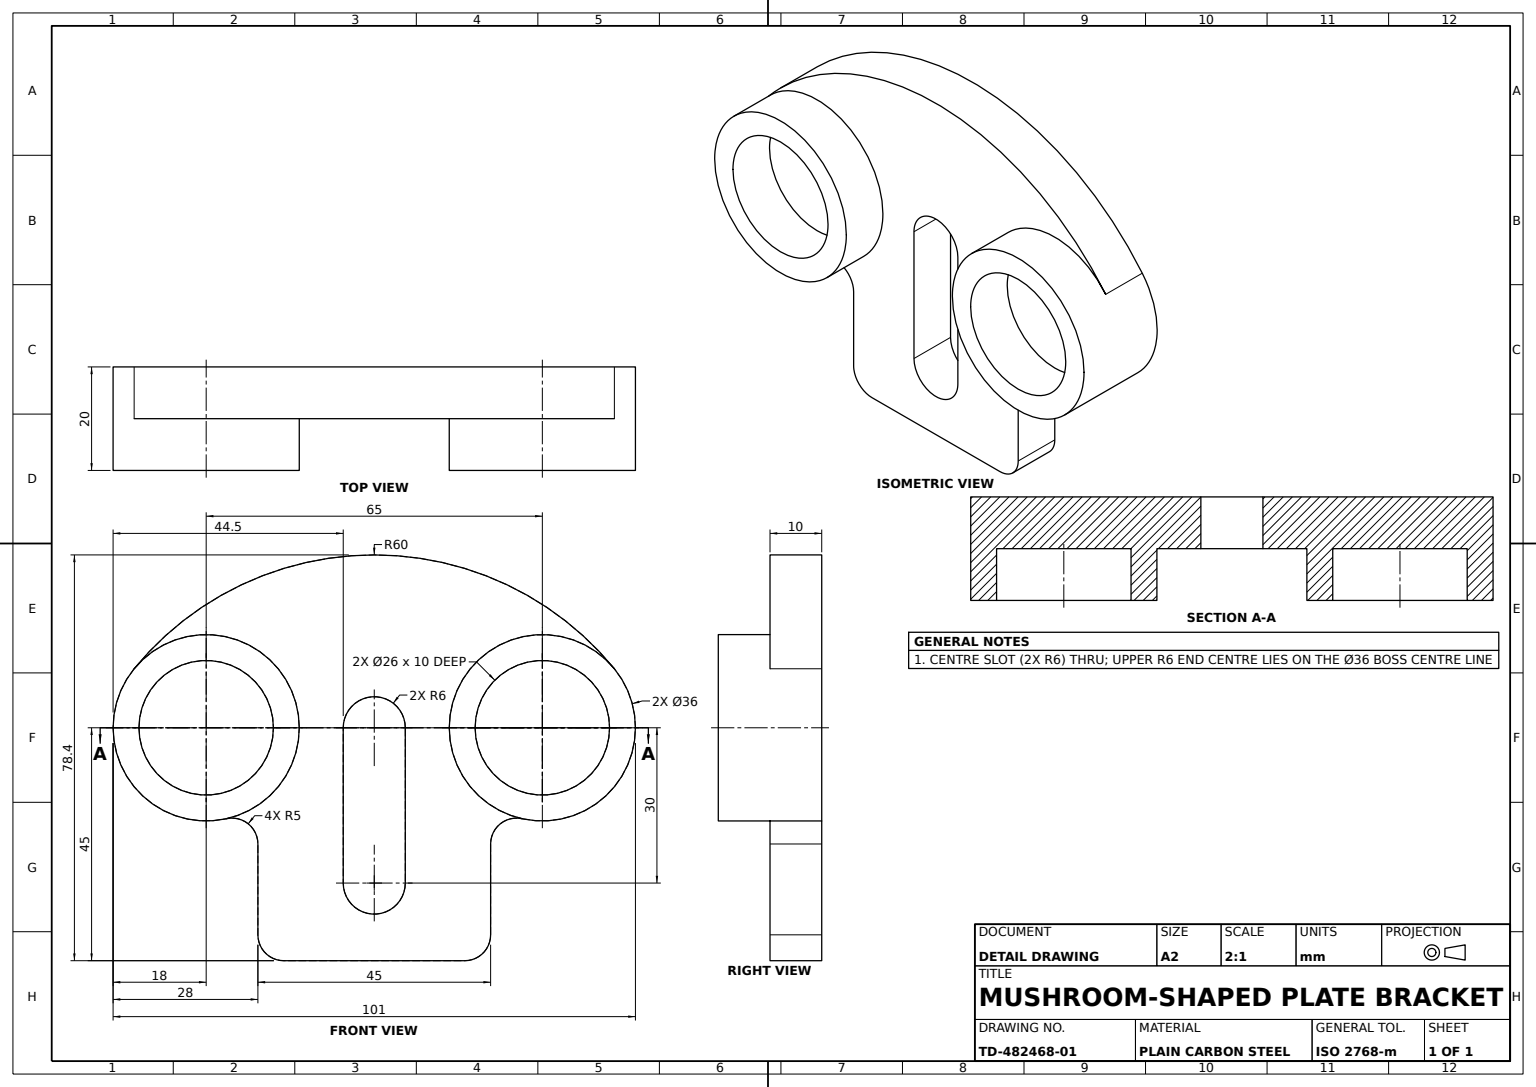
from build123d import *

# Parameters (mm, degrees)
LOBED_BASE_PLATE_DEPTH   = 10
ROUND_BOSSES_SKETCH_R    = 18
ROUND_BOSSES_2X_36_DEPTH = 10
BOSS_BORES_SKETCH_R      = 13
BOSS_BORES_2X_13_DEPTH   = 10
CENTER_SLOT_DEPTH        = 20


with BuildPart() as part:
    # Lobed Base Sketch → Lobed Base Plate (new body)
    with BuildSketch(Plane.XY):
        with BuildLine():
            Line((15, -45), (50, -45))
            ThreePointArc((50, -45), (53.535533906, -43.535533906), (55, -40))
            Line((55, -40), (55, -22.449944321))
            ThreePointArc((55, -22.449944321), (56.872283789, -18.548996833), (61.086956522, -17.569521642))
            ThreePointArc((61.086956522, -17.569521642), (80.32671412, -9.438847084), (78.928571429, 11.40153051))
            ThreePointArc((78.928571429, 11.40153051), (32.5, 33.396428811), (-13.928571429, 11.40153051))
            ThreePointArc((-13.928571429, 11.40153051), (-15.32671412, -9.438847084), (3.913043478, -17.569521642))
            ThreePointArc((3.913043478, -17.569521642), (8.127716211, -18.548996833), (10, -22.449944321))
            Line((10, -22.449944321), (10, -40))
            ThreePointArc((10, -40), (11.464466094, -43.535533906), (15, -45))
        make_face()
    extrude(amount=LOBED_BASE_PLATE_DEPTH)

    # Round Bosses Sketch → Round Bosses 2xØ36 (add)
    with BuildSketch(Plane.XY.offset(10)):
        with Locations(Location((0, 0, 0), (0, 0, 140.697224227))):
            Circle(ROUND_BOSSES_SKETCH_R)
        with Locations(Location((65, 0, 0), (0, 0, 257.444142201))):
            Circle(ROUND_BOSSES_SKETCH_R)
    extrude(amount=ROUND_BOSSES_2X_36_DEPTH)

    # Boss Bores Sketch → Boss Bores 2xØ13 (cut)
    with BuildSketch(Plane.XY.offset(20)):
        Circle(BOSS_BORES_SKETCH_R)
        with Locations((65, 0)):
            Circle(BOSS_BORES_SKETCH_R)
    extrude(amount=-BOSS_BORES_2X_13_DEPTH, mode=Mode.SUBTRACT)

    # Center Slot Sketch → Center Slot (cut)
    with BuildSketch(Plane.XY.offset(10)):
        with BuildLine():
            Line((26.5, 0), (26.5, -30))
            ThreePointArc((26.5, -30), (32.5, -36), (38.5, -30))
            Line((38.5, -30), (38.5, 0))
            ThreePointArc((38.5, 0), (32.5, 6), (26.5, 0))
        make_face()
    extrude(amount=-CENTER_SLOT_DEPTH, mode=Mode.SUBTRACT)


solid = part.part
